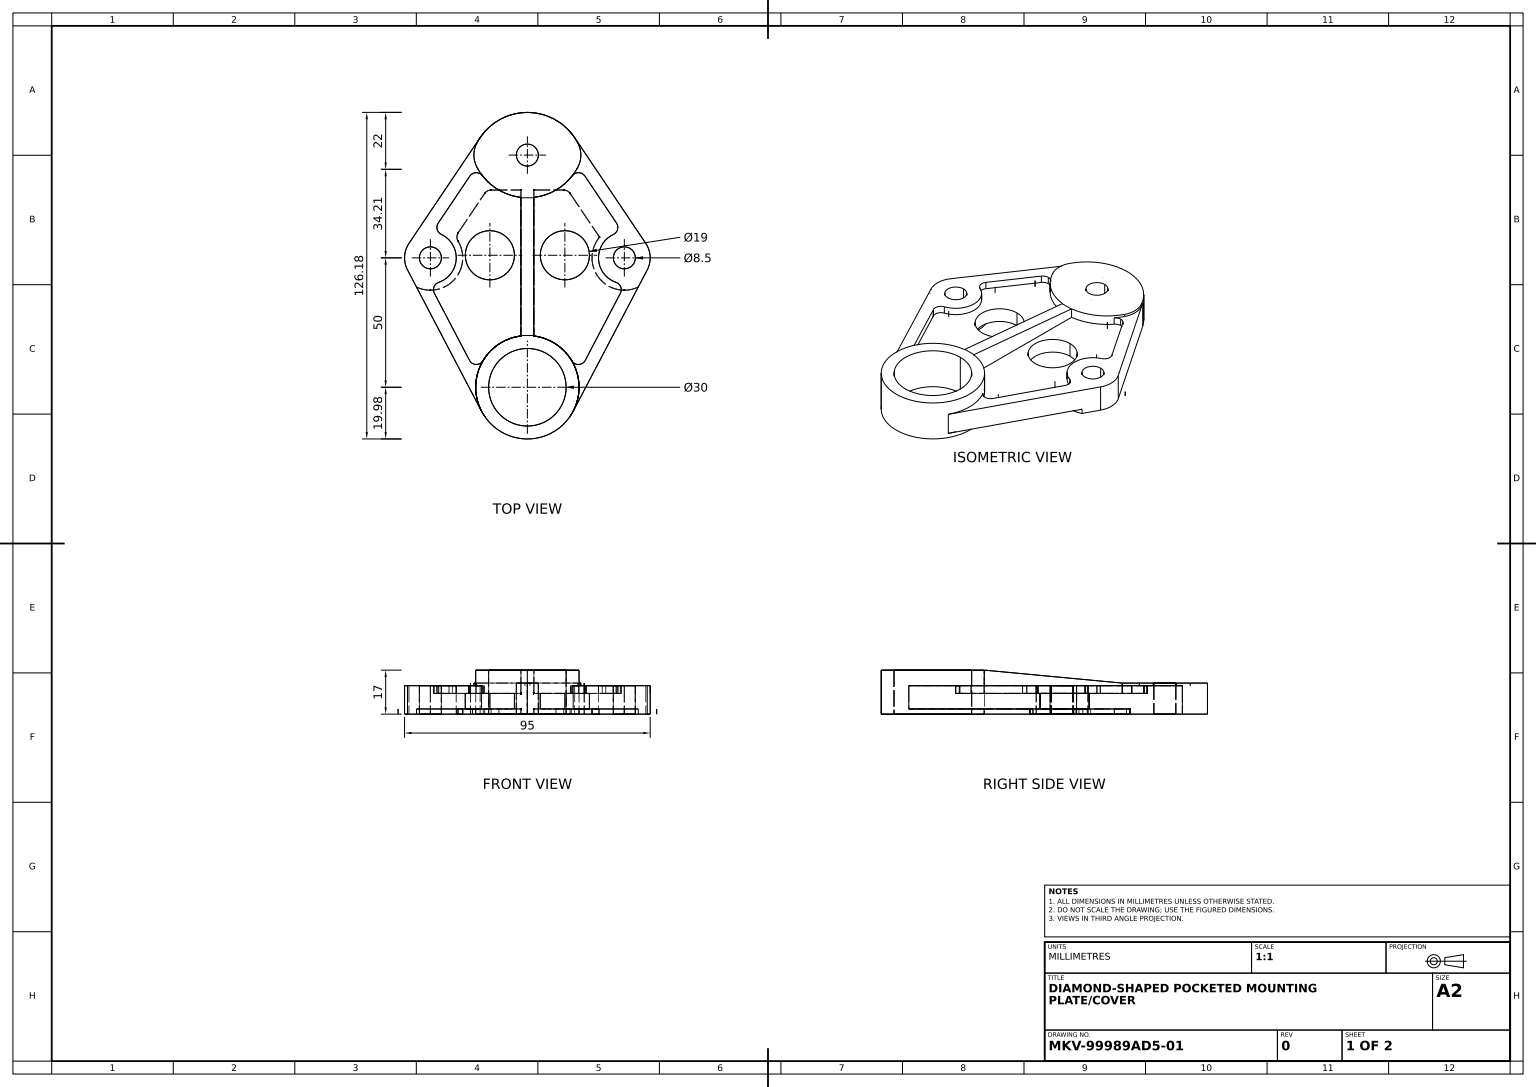
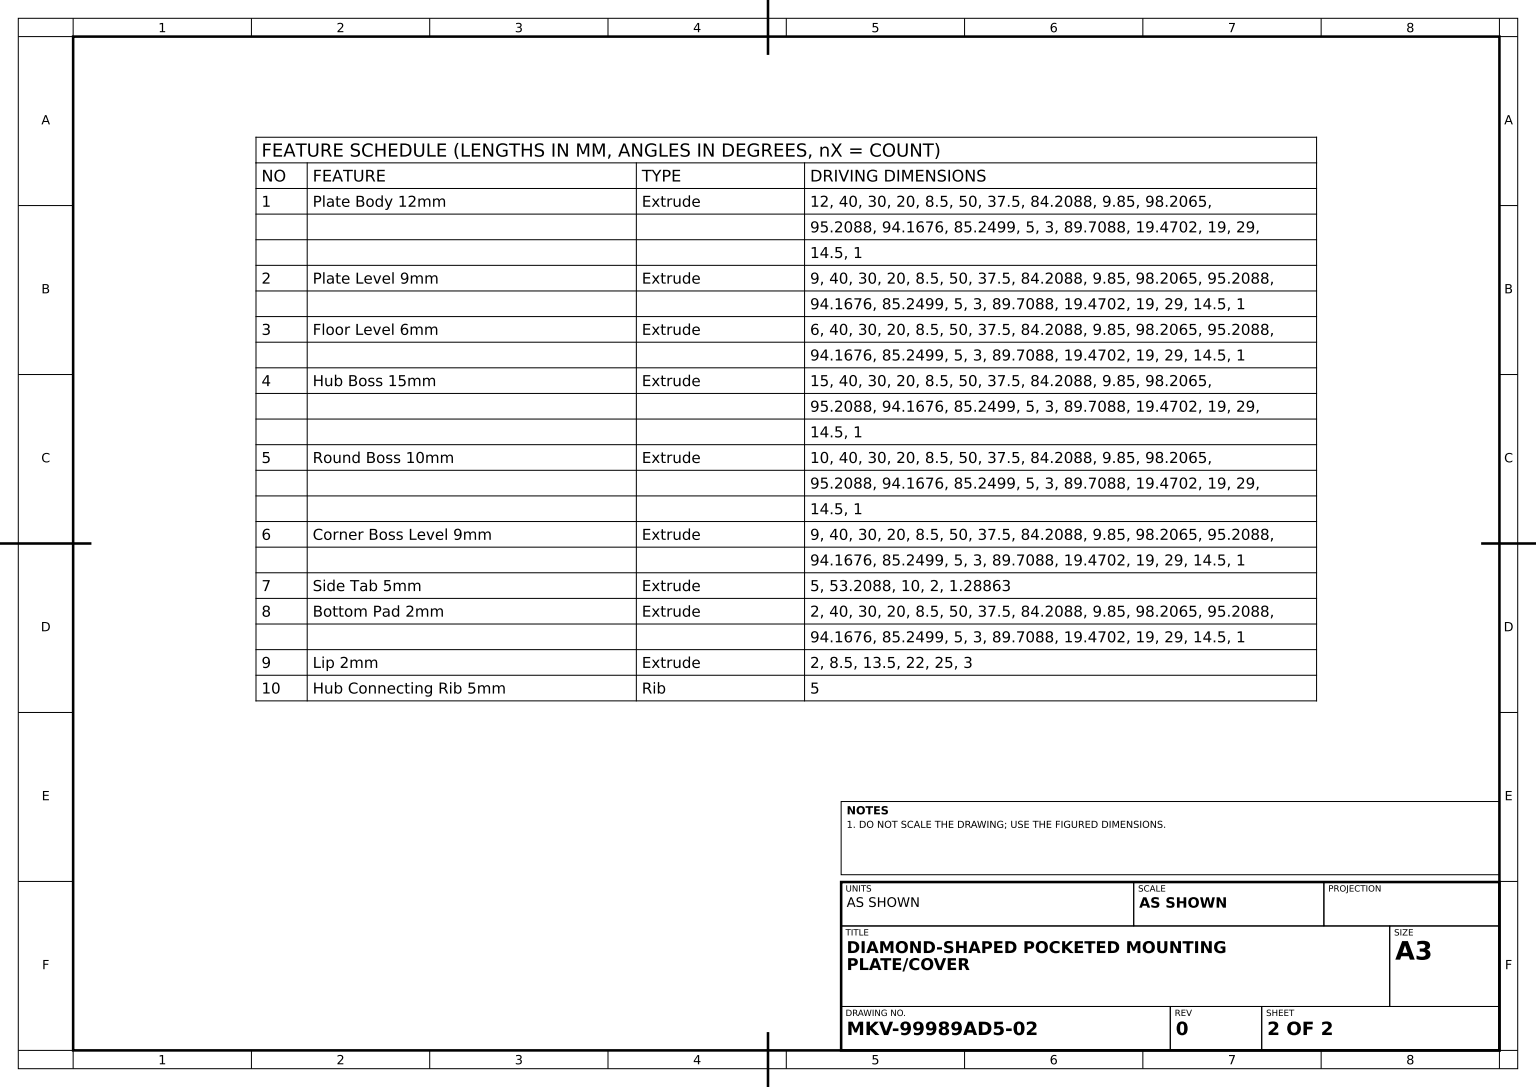
from build123d import *
from build123d.topology import SkipClean

# Parameters (mm, degrees)
PLATE_CONTOURS_SKETCH_R      = 20
PLATE_CONTOURS_SKETCH_R_2    = 15
PLATE_BODY_12MM_DEPTH        = 12
SKETCH1_3_R                  = 4.25
PLATE_LEVEL_9MM_DEPTH        = 9
SKETCH1_4_R                  = 10
SKETCH1_4_R_2                = 4.25
SKETCH1_4_R_3                = 9.5
FLOOR_LEVEL_6MM_DEPTH        = 6
SKETCH1_5_R                  = 20
SKETCH1_5_R_2                = 15
HUB_BOSS_15MM_DEPTH          = 15
SKETCH1_6_R                  = 4.25
ROUND_BOSS_10MM_DEPTH        = 10
SKETCH1_7_R                  = 10
SKETCH1_7_R_2                = 4.25
CORNER_BOSS_LEVEL_9MM_DEPTH  = 9
SIDE_TAB_5MM_DEPTH           = 2.5
BOTTOM_START                 = -2
SKETCH1_8_R                  = 20
SKETCH1_8_R_2                = 15
BOTTOM_PAD_2MM_DEPTH         = 2
LIP_START                    = 2
LIP_PROFILE_SKETCH_R         = 4.25
LIP_2MM_DEPTH                = 2
HUB_CONNECTING_RIB_5MM_REACH = 119.582
HUB_RIB_PATH_SKETCH_WALLS_W  = 5
HUB_RIB_PATH_SKETCH_WALLS_H  = 293.373025838


with BuildPart() as part:
    # Plate Contours Sketch → Plate Body 12mm (new body)
    with BuildSketch(Plane(origin=(0, 0, 0), x_dir=(1, 0, 0), z_dir=(0, 1, 0))):
        with Locations(Location((0, 0, 0), (0, 0, 270))):
            Circle(PLATE_CONTOURS_SKETCH_R)
        with Locations(Location((0, 0, 0), (0, 0, 270))):
            Circle(PLATE_CONTOURS_SKETCH_R_2, mode=Mode.SUBTRACT)
    extrude(amount=PLATE_BODY_12MM_DEPTH)



with BuildPart() as body_2:
    # Sketch1_3 → Plate Level 9mm (new body)
    with BuildSketch(Plane(origin=(0, 0, 0), x_dir=(1, 0, 0), z_dir=(0, 1, 0))):
        with BuildLine():
            ThreePointArc((19.616863963, 94.1676298), (20.683858962, 89.708782064), (19.616863963, 85.249934327))
            ThreePointArc((19.616863963, 85.249934327), (0, 73.208782064), (-19.616863963, 85.249934327))
            ThreePointArc((-19.616863963, 85.249934327), (-20.683858962, 89.708782064), (-19.616863963, 94.1676298))
            ThreePointArc((-19.616863963, 94.1676298), (0, 106.208782064), (19.616863963, 94.1676298))
        make_face()
        with Locations(Location((0, 89.708782064, 0), (0, 0, 270))):
            Circle(SKETCH1_3_R, mode=Mode.SUBTRACT)
    extrude(amount=PLATE_LEVEL_9MM_DEPTH)


with BuildPart() as part_1:
    add(part.part)

    add(body_2.part)  # Floor Level 6mm merges body 2
    # Sketch1_4 → Floor Level 6mm (add)
    # profile 1 of 7: a face of its own
    with BuildSketch(Plane(origin=(0, 0, 0), x_dir=(1, 0, 0), z_dir=(0, 1, 0))):
        with BuildLine():
            ThreePointArc((-34.275175703, 40.5342455), (-41.207509883, 40.712676894), (-46.356936115, 45.357297914))
            Line((-46.356936115, 45.357297914), (-17.713872229, -9.285404172))
            ThreePointArc((-17.713872229, -9.285404172), (-19.992079916, 0.562797133), (-17.163445775, 10.26723571))
            ThreePointArc((-17.163445775, 10.26723571), (-19.822382211, 8.808509079), (-22.395043476, 10.414510441))
            Line((-22.395043476, 10.414510441), (-35.964809248, 36.301708524))
            ThreePointArc((-35.964809248, 36.301708524), (-36.093925346, 38.806772115), (-34.275175703, 40.5342455))
        make_face()
    # profile 2 of 7: a face of its own
    with BuildSketch(Plane(origin=(0, 0, 0), x_dir=(1, 0, 0), z_dir=(0, 1, 0))):
        with Locations((-37.5, 50)):
            Circle(SKETCH1_4_R)
        with Locations(Location((-37.5, 50, 0), (0, 0, 270))):
            Circle(SKETCH1_4_R_2, mode=Mode.SUBTRACT)
    # profile 3 of 7: a face of its own
    with BuildSketch(Plane(origin=(0, 0, 0), x_dir=(1, 0, 0), z_dir=(0, 1, 0))):
        with BuildLine():
            Line((-18.248896479, 96.496083529), (-45.794952945, 55.58513703))
            ThreePointArc((-45.794952945, 55.58513703), (-40.167652212, 59.637615456), (-33.257501674, 59.055451836))
            ThreePointArc((-33.257501674, 59.055451836), (-34.876036813, 60.971791723), (-34.47323806, 63.447628496))
            Line((-34.47323806, 63.447628496), (-22.26076094, 81.585397097))
            ThreePointArc((-22.26076094, 81.585397097), (-19.871166838, 82.908225614), (-17.39960205, 81.745727117))
            ThreePointArc((-17.39960205, 81.745727117), (-18.590980503, 83.445472839), (-19.616863963, 85.249934327))
            ThreePointArc((-19.616863963, 85.249934327), (-20.683858962, 89.708782064), (-19.616863963, 94.1676298))
            ThreePointArc((-19.616863963, 94.1676298), (-18.968641956, 95.352866698), (-18.248896479, 96.496083529))
        make_face()
    # profile 4 of 7: a face of its own
    with BuildSketch(Plane(origin=(0, 0, 0), x_dir=(1, 0, 0), z_dir=(0, 1, 0))):
        with BuildLine():
            Line((45.794952945, 55.58513703), (18.248896479, 96.496083529))
            ThreePointArc((18.248896479, 96.496083529), (18.968641956, 95.352866698), (19.616863963, 94.1676298))
            ThreePointArc((19.616863963, 94.1676298), (20.683858962, 89.708782064), (19.616863963, 85.249934327))
            ThreePointArc((19.616863963, 85.249934327), (18.590980503, 83.445472839), (17.39960205, 81.745727117))
            ThreePointArc((17.39960205, 81.745727117), (19.871166838, 82.908225614), (22.26076094, 81.585397097))
            Line((22.26076094, 81.585397097), (34.47323806, 63.447628496))
            ThreePointArc((34.47323806, 63.447628496), (34.876036813, 60.971791723), (33.257501674, 59.055451836))
            ThreePointArc((33.257501674, 59.055451836), (40.167652212, 59.637615456), (45.794952945, 55.58513703))
        make_face()
    # profile 5 of 7: a face of its own
    with BuildSketch(Plane(origin=(0, 0, 0), x_dir=(1, 0, 0), z_dir=(0, 1, 0))):
        with Locations((37.5, 50)):
            Circle(SKETCH1_4_R)
        with Locations(Location((37.5, 50, 0), (0, 0, 270))):
            Circle(SKETCH1_4_R_2, mode=Mode.SUBTRACT)
    # profile 6 of 7: a face of its own
    with BuildSketch(Plane(origin=(0, 0, 0), x_dir=(1, 0, 0), z_dir=(0, 1, 0))):
        with BuildLine():
            ThreePointArc((20, 0), (19.420059791, -4.781346851), (17.713872229, -9.285404172))
            Line((17.713872229, -9.285404172), (46.356936115, 45.357297914))
            ThreePointArc((46.356936115, 45.357297914), (41.207509883, 40.712676894), (34.275175703, 40.5342455))
            ThreePointArc((34.275175703, 40.5342455), (36.093925346, 38.806772115), (35.964809248, 36.301708524))
            Line((35.964809248, 36.301708524), (22.395043476, 10.414510441))
            ThreePointArc((22.395043476, 10.414510441), (19.822382211, 8.808509079), (17.163445775, 10.26723571))
            ThreePointArc((17.163445775, 10.26723571), (19.277822951, 5.325931116), (20, 0))
        make_face()
    # profile 7 of 7: a face of its own
    with BuildSketch(Plane(origin=(0, 0, 0), x_dir=(1, 0, 0), z_dir=(0, 1, 0))):
        with BuildLine():
            ThreePointArc((-34.47323806, 63.447628496), (-34.876036813, 60.971791723), (-33.257501674, 59.055451836))
            ThreePointArc((-33.257501674, 59.055451836), (-29.061250589, 55.365399181), (-27.5, 50))
            ThreePointArc((-27.5, 50), (-29.368326034, 44.179701166), (-34.275175703, 40.5342455))
            ThreePointArc((-34.275175703, 40.5342455), (-36.093925346, 38.806772115), (-35.964809248, 36.301708524))
            Line((-35.964809248, 36.301708524), (-22.395043476, 10.414510441))
            ThreePointArc((-22.395043476, 10.414510441), (-19.822382211, 8.808509079), (-17.163445775, 10.26723571))
            ThreePointArc((-17.163445775, 10.26723571), (0, 20), (17.163445775, 10.26723571))
            ThreePointArc((17.163445775, 10.26723571), (19.822382211, 8.808509079), (22.395043476, 10.414510441))
            Line((22.395043476, 10.414510441), (35.964809248, 36.301708524))
            ThreePointArc((35.964809248, 36.301708524), (36.093925346, 38.806772115), (34.275175703, 40.5342455))
            ThreePointArc((34.275175703, 40.5342455), (27.515061451, 49.451363348), (33.257501674, 59.055451836))
            ThreePointArc((33.257501674, 59.055451836), (34.876036813, 60.971791723), (34.47323806, 63.447628496))
            Line((34.47323806, 63.447628496), (22.26076094, 81.585397097))
            ThreePointArc((22.26076094, 81.585397097), (19.871166838, 82.908225614), (17.39960205, 81.745727117))
            ThreePointArc((17.39960205, 81.745727117), (0, 73.208782064), (-17.39960205, 81.745727117))
            ThreePointArc((-17.39960205, 81.745727117), (-19.871166838, 82.908225614), (-22.26076094, 81.585397097))
            Line((-22.26076094, 81.585397097), (-34.47323806, 63.447628496))
        make_face()
        with Locations(Location((-14.5, 51, 0), (0, 0, 270))):
            Circle(SKETCH1_4_R_3, mode=Mode.SUBTRACT)
        with Locations(Location((14.5, 51, 0), (0, 0, 270))):
            Circle(SKETCH1_4_R_3, mode=Mode.SUBTRACT)
    extrude(amount=FLOOR_LEVEL_6MM_DEPTH)

    # Sketch1_5 → Hub Boss 15mm (add)
    with BuildSketch(Plane(origin=(0, 0, 0), x_dir=(1, 0, 0), z_dir=(0, 1, 0))):
        with Locations(Location((0, 0, 0), (0, 0, 332.336998576))):
            Circle(SKETCH1_5_R)
        with Locations(Location((0, 0, 0), (0, 0, 270))):
            Circle(SKETCH1_5_R_2, mode=Mode.SUBTRACT)
    extrude(amount=HUB_BOSS_15MM_DEPTH)

    # Sketch1_6 → Round Boss 10mm (add)
    with BuildSketch(Plane(origin=(0, 0, 0), x_dir=(1, 0, 0), z_dir=(0, 1, 0))):
        with BuildLine():
            ThreePointArc((19.616863963, 94.1676298), (20.683858962, 89.708782064), (19.616863963, 85.249934327))
            ThreePointArc((19.616863963, 85.249934327), (0, 73.208782064), (-19.616863963, 85.249934327))
            ThreePointArc((-19.616863963, 85.249934327), (-20.683858962, 89.708782064), (-19.616863963, 94.1676298))
            ThreePointArc((-19.616863963, 94.1676298), (0, 106.208782064), (19.616863963, 94.1676298))
        make_face()
        with Locations(Location((0, 89.708782064, 0), (0, 0, 270))):
            Circle(SKETCH1_6_R, mode=Mode.SUBTRACT)
    extrude(amount=ROUND_BOSS_10MM_DEPTH)

    # Sketch1_7 → Corner Boss Level 9mm (add)
    # profile 1 of 6: a face of its own
    with BuildSketch(Plane(origin=(0, 0, 0), x_dir=(1, 0, 0), z_dir=(0, 1, 0))):
        with BuildLine():
            ThreePointArc((-34.275175703, 40.5342455), (-41.207509883, 40.712676894), (-46.356936115, 45.357297914))
            Line((-46.356936115, 45.357297914), (-17.713872229, -9.285404172))
            ThreePointArc((-17.713872229, -9.285404172), (-19.992079916, 0.562797133), (-17.163445775, 10.26723571))
            ThreePointArc((-17.163445775, 10.26723571), (-19.822382211, 8.808509079), (-22.395043476, 10.414510441))
            Line((-22.395043476, 10.414510441), (-35.964809248, 36.301708524))
            ThreePointArc((-35.964809248, 36.301708524), (-36.093925346, 38.806772115), (-34.275175703, 40.5342455))
        make_face()
    # profile 2 of 6: a face of its own
    with BuildSketch(Plane(origin=(0, 0, 0), x_dir=(1, 0, 0), z_dir=(0, 1, 0))):
        with Locations((-37.5, 50)):
            Circle(SKETCH1_7_R)
        with Locations(Location((-37.5, 50, 0), (0, 0, 270))):
            Circle(SKETCH1_7_R_2, mode=Mode.SUBTRACT)
    # profile 3 of 6: a face of its own
    with BuildSketch(Plane(origin=(0, 0, 0), x_dir=(1, 0, 0), z_dir=(0, 1, 0))):
        with BuildLine():
            Line((-18.248896479, 96.496083529), (-45.794952945, 55.58513703))
            ThreePointArc((-45.794952945, 55.58513703), (-40.167652212, 59.637615456), (-33.257501674, 59.055451836))
            ThreePointArc((-33.257501674, 59.055451836), (-34.876036813, 60.971791723), (-34.47323806, 63.447628496))
            Line((-34.47323806, 63.447628496), (-22.26076094, 81.585397097))
            ThreePointArc((-22.26076094, 81.585397097), (-19.871166838, 82.908225614), (-17.39960205, 81.745727117))
            ThreePointArc((-17.39960205, 81.745727117), (-18.590980503, 83.445472839), (-19.616863963, 85.249934327))
            ThreePointArc((-19.616863963, 85.249934327), (-20.683858962, 89.708782064), (-19.616863963, 94.1676298))
            ThreePointArc((-19.616863963, 94.1676298), (-18.968641956, 95.352866698), (-18.248896479, 96.496083529))
        make_face()
    # profile 4 of 6: a face of its own
    with BuildSketch(Plane(origin=(0, 0, 0), x_dir=(1, 0, 0), z_dir=(0, 1, 0))):
        with BuildLine():
            Line((45.794952945, 55.58513703), (18.248896479, 96.496083529))
            ThreePointArc((18.248896479, 96.496083529), (18.968641956, 95.352866698), (19.616863963, 94.1676298))
            ThreePointArc((19.616863963, 94.1676298), (20.683858962, 89.708782064), (19.616863963, 85.249934327))
            ThreePointArc((19.616863963, 85.249934327), (18.590980503, 83.445472839), (17.39960205, 81.745727117))
            ThreePointArc((17.39960205, 81.745727117), (19.871166838, 82.908225614), (22.26076094, 81.585397097))
            Line((22.26076094, 81.585397097), (34.47323806, 63.447628496))
            ThreePointArc((34.47323806, 63.447628496), (34.876036813, 60.971791723), (33.257501674, 59.055451836))
            ThreePointArc((33.257501674, 59.055451836), (40.167652212, 59.637615456), (45.794952945, 55.58513703))
        make_face()
    # profile 5 of 6: a face of its own
    with BuildSketch(Plane(origin=(0, 0, 0), x_dir=(1, 0, 0), z_dir=(0, 1, 0))):
        with Locations((37.5, 50)):
            Circle(SKETCH1_7_R)
        with Locations(Location((37.5, 50, 0), (0, 0, 270))):
            Circle(SKETCH1_7_R_2, mode=Mode.SUBTRACT)
    # profile 6 of 6: a face of its own
    with BuildSketch(Plane(origin=(0, 0, 0), x_dir=(1, 0, 0), z_dir=(0, 1, 0))):
        with BuildLine():
            ThreePointArc((20, 0), (19.420059791, -4.781346851), (17.713872229, -9.285404172))
            Line((17.713872229, -9.285404172), (46.356936115, 45.357297914))
            ThreePointArc((46.356936115, 45.357297914), (41.207509883, 40.712676894), (34.275175703, 40.5342455))
            ThreePointArc((34.275175703, 40.5342455), (36.093925346, 38.806772115), (35.964809248, 36.301708524))
            Line((35.964809248, 36.301708524), (22.395043476, 10.414510441))
            ThreePointArc((22.395043476, 10.414510441), (19.822382211, 8.808509079), (17.163445775, 10.26723571))
            ThreePointArc((17.163445775, 10.26723571), (19.277822951, 5.325931116), (20, 0))
        make_face()
    extrude(amount=CORNER_BOSS_LEVEL_9MM_DEPTH)

    # Side Tab Sketch → Side Tab 5mm (add, symmetric)
    with BuildSketch(Plane(origin=(0, 0, 0), x_dir=(0, 0, -1), z_dir=(1, 0, 0))):
        Polygon((20, 15), (73.208782064, 10), (74.497408644, 10), (74.497408644, 5), (73.208782064, 5), (18, 5), (18, 15), align=None)
    extrude(amount=SIDE_TAB_5MM_DEPTH, both=True)

    # Sketch1_8 → Bottom Pad 2mm (add)
    with BuildSketch(Plane(origin=(0, 0, 0), x_dir=(1, 0, 0), z_dir=(0, 1, 0)).offset(BOTTOM_START)):
        with Locations(Location((0, 0, 0), (0, 0, 97.180755781))):
            Circle(SKETCH1_8_R)
        with Locations(Location((0, 0, 0), (0, 0, 270))):
            Circle(SKETCH1_8_R_2, mode=Mode.SUBTRACT)
    extrude(amount=BOTTOM_PAD_2MM_DEPTH)

    # Lip Profile Sketch → Lip 2mm (add)
    with SkipClean():  # the faces are left unmerged after this step: merging them gives an invalid solid
        with BuildSketch(Plane.XZ.offset(LIP_START)):
            with BuildLine():
                ThreePointArc((-46.356936115, -45.357297914), (-47.484938549, -50.548636652), (-45.794952945, -55.58513703))
                Line((-45.794952945, -55.58513703), (-18.248896479, -96.496083529))
                ThreePointArc((-18.248896479, -96.496083529), (0, -106.208782064), (18.248896479, -96.496083529))
                Line((18.248896479, -96.496083529), (45.794952945, -55.58513703))
                ThreePointArc((45.794952945, -55.58513703), (47.484938549, -50.548636652), (46.356936115, -45.357297914))
                Line((46.356936115, -45.357297914), (42.87490955, -38.714595828))
                ThreePointArc((42.87490955, -38.714595828), (27.628438686, -42.33173571), (27.894602034, -57.999145574))
                Line((27.894602034, -57.999145574), (16.525516364, -74.884323173))
                ThreePointArc((16.525516364, -74.884323173), (15.446529802, -75.857047848), (14.037030481, -76.208782064))
                Line((14.037030481, -76.208782064), (-14.037030481, -76.208782064))
                ThreePointArc((-14.037030481, -76.208782064), (-15.446529802, -75.857047848), (-16.525516364, -74.884323173))
                Line((-16.525516364, -74.884323173), (-26.737782046, -59.717235446))
                ThreePointArc((-26.737782046, -59.717235446), (-27.248463448, -58.112373832), (-26.813948518, -56.485237369))
                ThreePointArc((-26.813948518, -56.485237369), (-28.22632854, -41.618531295), (-42.87490955, -38.714595828))
                Line((-42.87490955, -38.714595828), (-46.356936115, -45.357297914))
            make_face()
            with Locations(Location((0, -89.708782064, 0), (0, 0, 270))):
                Circle(LIP_PROFILE_SKETCH_R, mode=Mode.SUBTRACT)
            with Locations(Location((-37.5, -50, 0), (0, 0, 270))):
                Circle(LIP_PROFILE_SKETCH_R, mode=Mode.SUBTRACT)
            with Locations(Location((37.5, -50, 0), (0, 0, 270))):
                Circle(LIP_PROFILE_SKETCH_R, mode=Mode.SUBTRACT)
        extrude(amount=-LIP_2MM_DEPTH)

    # Hub Rib Path Sketch walls → Hub Connecting Rib 5mm (add, up to next)
    with BuildSketch(Plane.XZ.offset(2), mode=Mode.PRIVATE) as hub_connecting_rib_5mm_sk1:
        with Locations((0, -48.104391032)):
            Rectangle(HUB_RIB_PATH_SKETCH_WALLS_W, HUB_RIB_PATH_SKETCH_WALLS_H)
    hub_connecting_rib_5mm_tool1 = extrude(hub_connecting_rib_5mm_sk1.sketch, amount=-HUB_CONNECTING_RIB_5MM_REACH, mode=Mode.PRIVATE) - part_1.part
    add(hub_connecting_rib_5mm_tool1.solids().sort_by_distance((0, -2, -48.104391032))[0])


solid = part_1.part
